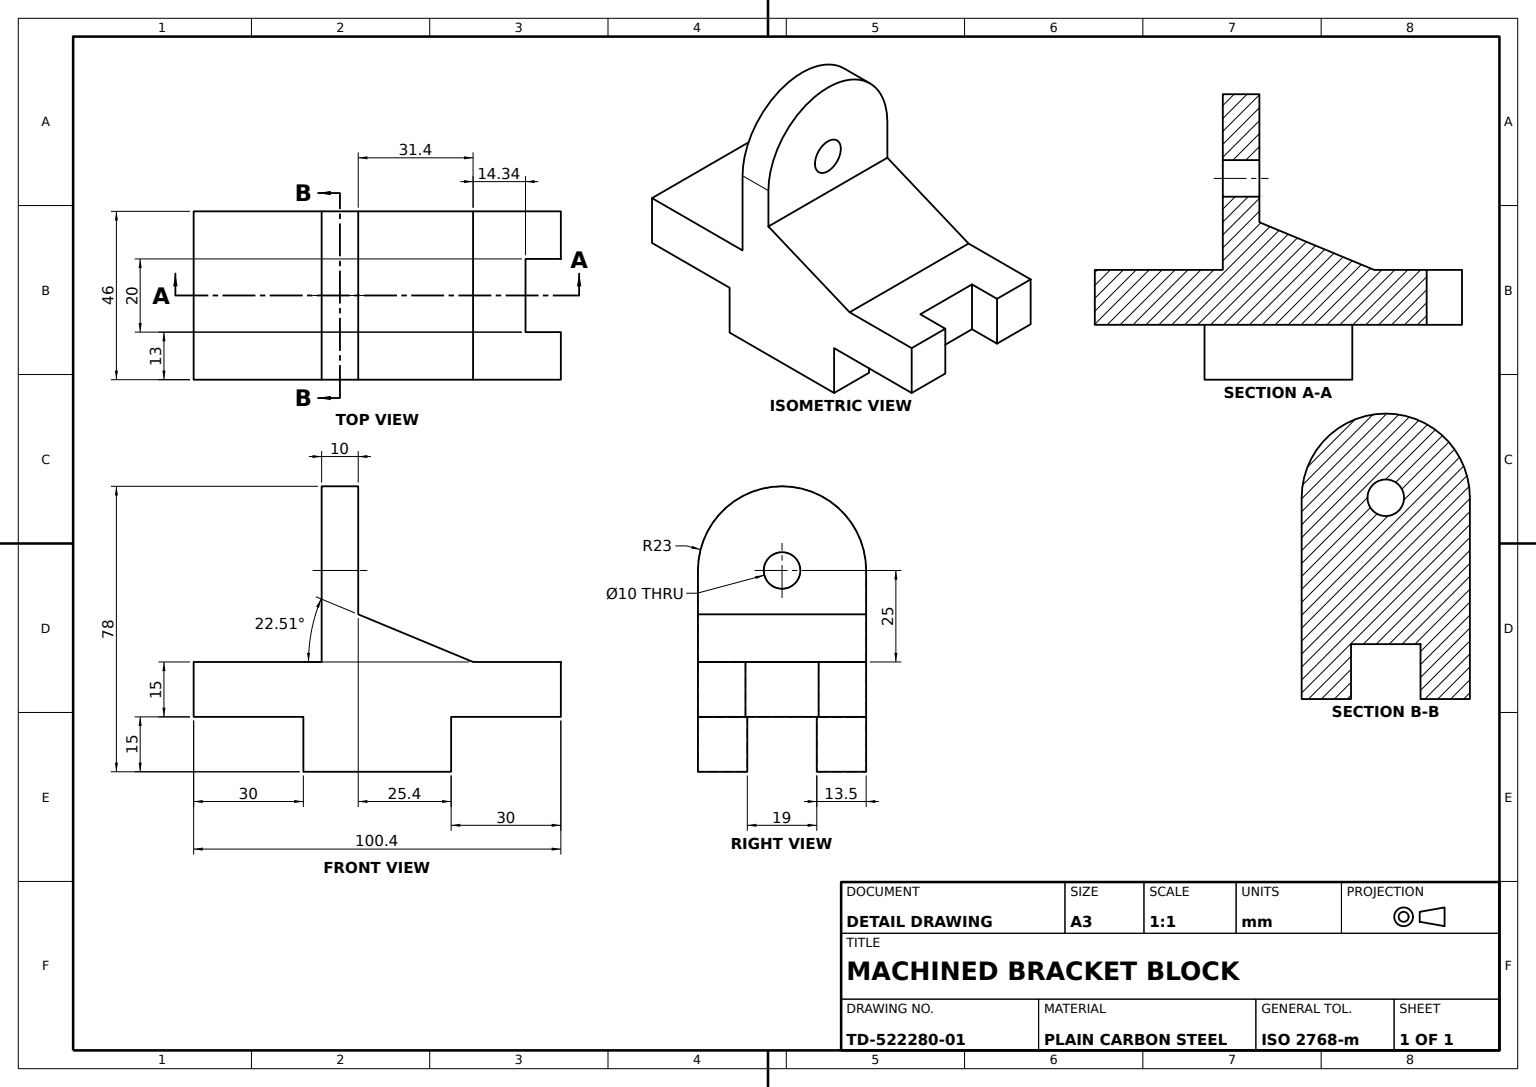
from build123d import *

# Parameters (mm, degrees)
BASE_BODY_DEPTH         = 46
SIDE_BLOCK_SKETCH_W     = 10
SIDE_BLOCK_SKETCH_H     = 25
SIDE_BLOCK_DEPTH        = 23
FRONT_BLOCK_DEPTH       = 23
LUG_DEPTH               = 10
LUG_EXTENSION_SKETCH_R  = 5
LUG_EXTENSION_DEPTH     = 10
PIN_HOLE_SKETCH_R       = 5
LUG_PIN_HOLE_DEPTH      = 10
SLOT_SKETCH_W           = 20
SLOT_SKETCH_H           = 19.323161221
SLOT_CUT_DEPTH          = 19
ANGLED_RELIEF_CUT_DEPTH = 81


with BuildPart() as part:
    # Base Profile Sketch → Base Body (new body)
    with BuildSketch(Plane(origin=(0, 0, 0), x_dir=(0, 0, -1), z_dir=(1, 0, 0))):
        Polygon((50.202309924, 0), (-50.202309924, 0), (-50.202309924, -15), (-20.202309924, -15), (-20.202309924, -30), (20.202309924, -30), (20.202309924, -15), (50.202309924, -15), align=None)
    extrude(amount=BASE_BODY_DEPTH)

    # Side Block Sketch → Side Block (add, symmetric)
    with BuildSketch(Plane(origin=(23, 0, 0), x_dir=(0, 0, -1), z_dir=(1, 0, 0))):
        with Locations((-10.202309924, 12.5)):
            Rectangle(SIDE_BLOCK_SKETCH_W, SIDE_BLOCK_SKETCH_H)
    extrude(amount=SIDE_BLOCK_DEPTH, both=True)

    # Front Block Sketch → Front Block (add, symmetric)
    with BuildSketch(Plane(origin=(23, 0, 0), x_dir=(0, 0, -1), z_dir=(1, 0, 0))):
        Polygon((-5.202309924, 13.015188061), (26.202309924, 0), (-5.202309924, 0), (-5.202309924, 13), align=None)
    extrude(amount=FRONT_BLOCK_DEPTH, both=True)

    # Lug Sketch → Lug (add)
    with BuildSketch(Plane(origin=(0, 0, 5.202309924), x_dir=(-1, 0, 0), z_dir=(0, 0, -1))):
        with BuildLine():
            ThreePointArc((-33, 25), (-23, 35), (-13, 25))
            Line((-13, 25), (0, 25))
            ThreePointArc((0, 25), (-23, 48), (-46, 25))
            Line((-46, 25), (-33, 25))
        make_face()
    extrude(amount=-LUG_DEPTH)

    # Lug Extension Sketch → Lug Extension (add)
    with BuildSketch(Plane(origin=(0, 0, 5.202309924), x_dir=(-1, 0, 0), z_dir=(0, 0, -1))):
        with Locations((-23, 25)):
            Circle(LUG_EXTENSION_SKETCH_R)
        with BuildLine():
            Line((-13, 25), (-33, 25))
            ThreePointArc((-33, 25), (-23, 35), (-13, 25))
        make_face()
        with BuildLine():
            ThreePointArc((-28, 25), (-23, 20), (-18, 25))
            Line((-18, 25), (-28, 25))
        make_face()
        with BuildLine():
            Line((-28, 25), (-18, 25))
            ThreePointArc((-18, 25), (-23, 30), (-28, 25))
        make_face()
    extrude(amount=-LUG_EXTENSION_DEPTH)

    # Pin Hole Sketch → Lug Pin Hole (cut)
    with BuildSketch(Plane(origin=(0, 0, 5.202309924), x_dir=(-1, 0, 0), z_dir=(0, 0, -1))):
        with Locations((-23, 25)):
            Circle(PIN_HOLE_SKETCH_R)
    extrude(amount=-LUG_PIN_HOLE_DEPTH, mode=Mode.SUBTRACT)

    # Slot Sketch → Slot Cut (cut)
    with BuildSketch(Plane(origin=(0, 0, 0), x_dir=(1, 0, 0), z_dir=(0, 1, 0))):
        with Locations((23, 50.202309924)):
            Rectangle(SLOT_SKETCH_W, SLOT_SKETCH_H)
    extrude(amount=-SLOT_CUT_DEPTH, mode=Mode.SUBTRACT)

    # Angled Cut Sketch → Angled Relief Cut (cut)
    with BuildSketch(Plane(origin=(0, 0, -20.202309924), x_dir=(-1, 0, 0), z_dir=(0, 0, -1))):
        Polygon((-23, -15), (-32.5, -15), (-32.5, -32.214795119), (-13.5, -32.214795119), (-13.5, -15), align=None)
    extrude(amount=-ANGLED_RELIEF_CUT_DEPTH, mode=Mode.SUBTRACT)


solid = part.part
